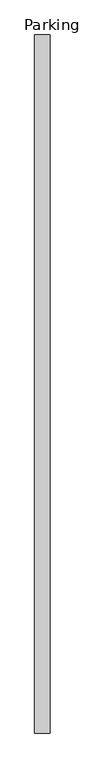
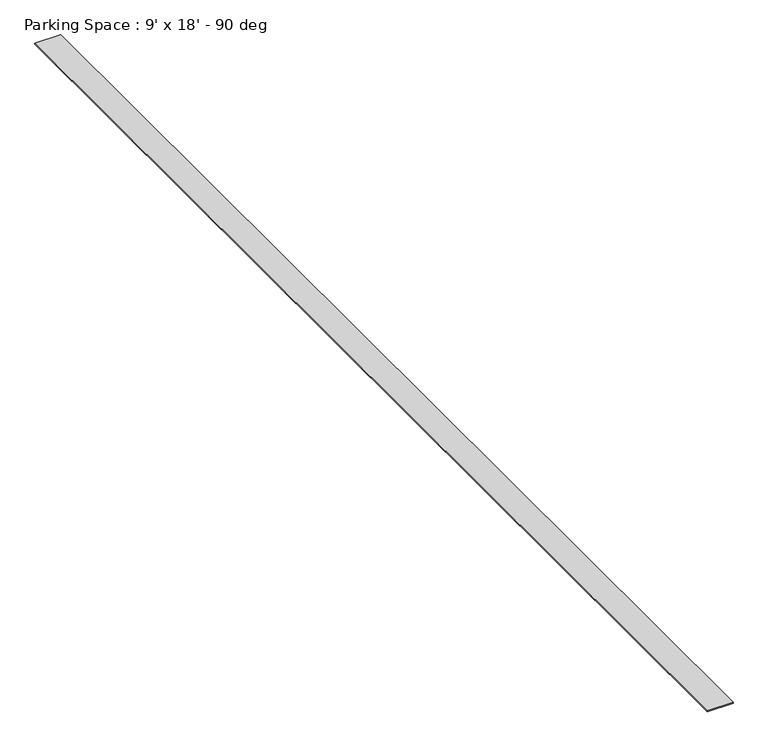
"""IFC4 building model written with IfcOpenShell, lengths in millimetres: proxy geometry, Parking Space : 9' x 18' - 90 deg."""

from ifc_helpers import new_model, si_unit, origin, origin_with_axes, place, context, project, spatial, polyline, outline, extrude, source, transform, mapped, element, save


def parking_space_9_x_18_90_deg_85bc4432(model_context):
    return source(origin(), model_context, "Body", "SweptSolid", [
        extrude(outline(polyline([(-50.8, 0.0), (50.8, 0.0), (50.8, -4572.0), (-50.8, -4572.0), (-50.8, 0.0)])), origin_with_axes(), (0.0, 0.0, 1.0), 3.175),
    ])


if __name__ == "__main__":
    model = new_model("IFC4")
    model_context = context("Model", 3, world=origin())
    ifc_project = project(units=[si_unit("LENGTHUNIT", "METRE", prefix="MILLI")], contexts=[model_context])
    site = spatial("IfcSite", under=ifc_project)
    building = spatial("IfcBuilding", under=site)
    placement = place(None, origin())
    parking_space_9_x_18_90_deg_shape = parking_space_9_x_18_90_deg_85bc4432(model_context)
    element("IfcBuildingElementProxy", 1, Name="Parking Space : 9' x 18' - 90 deg", ObjectType="Parking Space : 9' x 18' - 90 deg", at=placement, inside=building, context=model_context, shape_type="MappedRepresentation", body=[
        mapped(parking_space_9_x_18_90_deg_shape, transform((0.0, 0.0, 0.0), x_axis=(1.0, 0.0, 0.0), y_axis=(0.0, 1.0, 0.0), z_axis=(0.0, 0.0, 1.0))),
    ])
    save(model, "model.ifc")

# Revit data of these elements
# Type "Parking Space : 9' x 18' - 90 deg"
#   Angle = 90.00°
#   Parking Length = 18' - 0"
#   Parking Width = 9' - 0"
#   pl = 15' - 0"
#   pw = 8' - 0"
# Element 1 (IfcBuildingElementProxy, "Parking Space : 9' x 18' - 90 deg")
#   Materials on its faces: "Parking Stripe"
# Materials
#   "Parking Stripe": class "Paint", colour RGB 250 250 91, transparency 0
